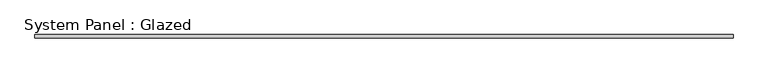
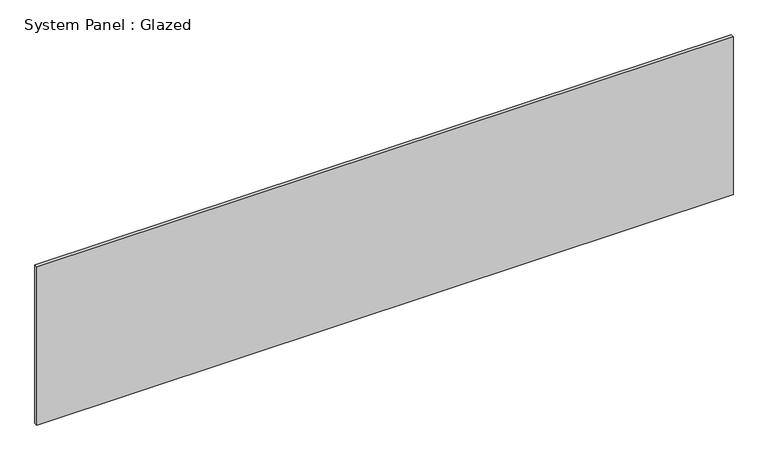
"""IFC4 building model written with IfcOpenShell, lengths in millimetres: plate geometry, System Panel : Glazed."""

from ifc_helpers import new_model, si_unit, origin, origin_with_axes, place, context, project, spatial, polyline, outline, extrude, source, transform, mapped, element, save


def system_panel_glazed_08041df1(model_context):
    return source(origin(), model_context, "Body", "SweptSolid", [
        extrude(outline(polyline([(2539.2990733, 19.05), (-2539.2990733, 19.05), (-2539.2990733, 44.45), (2539.2990733, 44.45), (2539.2990733, 19.05)])), origin_with_axes(), (0.0, 0.0, 1.0), 1219.2),
    ])


if __name__ == "__main__":
    model = new_model("IFC4")
    model_context = context("Model", 3, world=origin())
    ifc_project = project(units=[si_unit("LENGTHUNIT", "METRE", prefix="MILLI")], contexts=[model_context])
    site = spatial("IfcSite", under=ifc_project)
    building = spatial("IfcBuilding", under=site)
    placement = place(None, origin())
    system_panel_glazed_shape = system_panel_glazed_08041df1(model_context)
    element("IfcPlate", 1, ObjectType="System Panel : Glazed", at=placement, inside=building, context=model_context, shape_type="MappedRepresentation", body=[
        mapped(system_panel_glazed_shape, transform((0.0, 0.0, 0.0), x_axis=(1.0, 0.0, 0.0), y_axis=(0.0, 1.0, 0.0), z_axis=(0.0, 0.0, 1.0))),
    ])
    save(model, "model.ifc")

# Revit data of these elements
# Type "System Panel : Glazed"
#   Construction Type Id = "GSP4R"
#   Analytic Construction = "1/8 in Pilkington single glazing"
#   Visual Light Transmittance = 0.9
#   Solar Heat Gain Coefficient = 0.86
#   Heat Transfer Coefficient (U) = 1.18115 BTU/(h·ft²·°F)
# Element 1 (IfcPlate, "System Panel : Glazed")
#   Materials on its faces: "Glass"
# Materials
#   "Glass": class "Glass", colour RGB 0 128 192, transparency 0.75, Description = "Soda Lime Glass", Cost = 0
